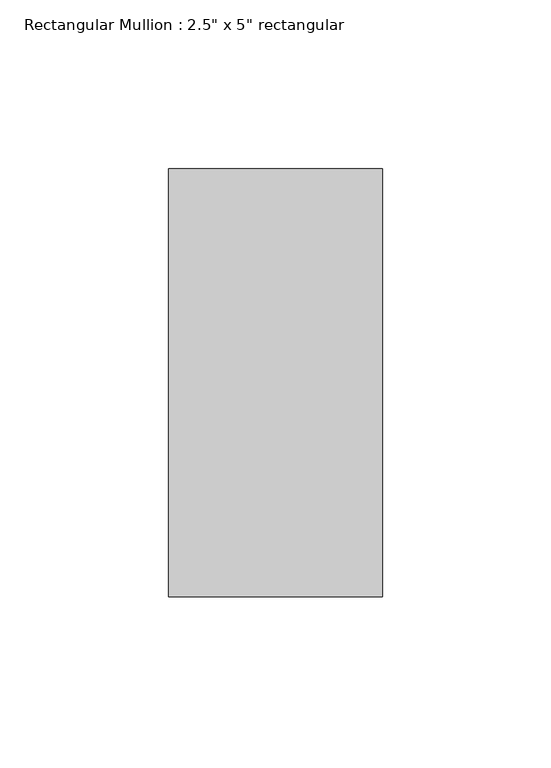
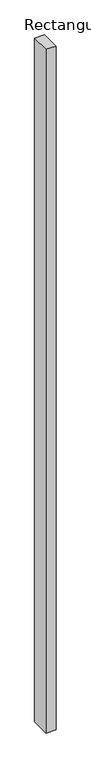
"""IFC4 building model written with IfcOpenShell, lengths in millimetres: member geometry."""

from ifc_helpers import new_model, si_unit, frame, origin, place, context, project, spatial, polyline, outline, extrude, source, transform, mapped, element, save


def member_0f997902(model_context):
    return source(origin(), model_context, "Body", "SweptSolid", [
        extrude(outline(polyline([(0.0, 63.5), (0.0, -63.5), (-63.5, -63.5), (-63.5, 63.5), (0.0, 63.5)])), frame((0.0, 0.0, -4660.9), z_axis=(0.0, 0.0, 1.0), x_axis=(1.0, 0.0, 0.0)), (0.0, 0.0, 1.0), 4660.9),
    ])


if __name__ == "__main__":
    model = new_model("IFC4")
    model_context = context("Model", 3, world=origin())
    ifc_project = project(units=[si_unit("LENGTHUNIT", "METRE", prefix="MILLI")], contexts=[model_context])
    site = spatial("IfcSite", under=ifc_project)
    building = spatial("IfcBuilding", under=site)
    placement = place(None, origin())
    member_shape = member_0f997902(model_context)
    element("IfcMember", 1, ObjectType="Rectangular Mullion : 2.5\" x 5\" rectangular", at=placement, inside=building, context=model_context, shape_type="MappedRepresentation", body=[
        mapped(member_shape, transform((0.0, 0.0, 0.0), x_axis=(1.0, 0.0, 0.0), y_axis=(0.0, 1.0, 0.0), z_axis=(0.0, 0.0, 1.0))),
    ])
    save(model, "model.ifc")

# Revit data of these elements
# Type "Rectangular Mullion : 2.5\" x 5\" rectangular"
#   built-in parameter 1007304 = 0.416667 (stored number, unit not read)
#   built-in parameter 1007301 = 0.104167 (stored number, unit not read)
#   built-in parameter 1007300 = 0.104167 (stored number, unit not read)
# Element 1 (IfcMember, "Rectangular Mullion : 2.5\" x 5\" rectangular")
#   Materials on its faces: "Aluminum"
# Materials
#   "Aluminum": class "Metal", colour RGB 247 247 247, transparency 0, Description = "Aluminum 6061", Cost = 0
